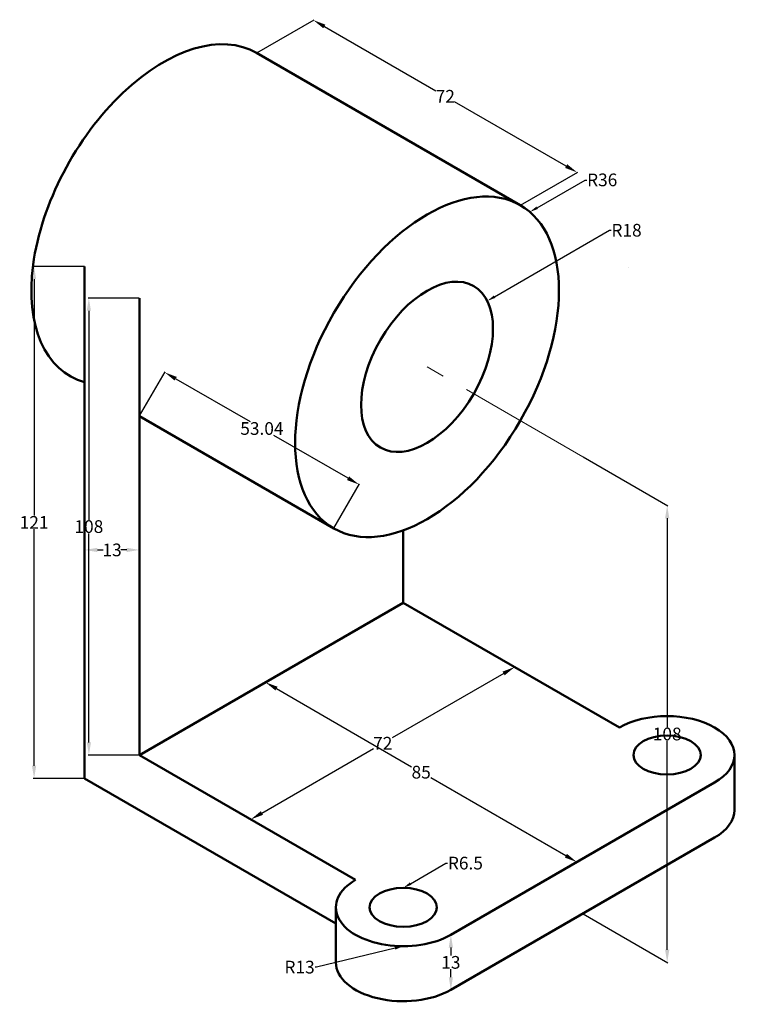
# Model space of a CAD drawing. Units: inches. Extents: x -9 to 160, y -49 to 184.
import ezdxf
from ezdxf import colors
from ezdxf.entities.mleader import LeaderData, LeaderLine
from ezdxf.math import Vec2, Vec3

# ---------------------------------------------------------------- set-up
doc = ezdxf.new("R2010")
doc.units = ezdxf.units.IN
doc.header["$MEASUREMENT"] = 0
doc.linetypes.add('CENTER', pattern=[50.8, 31.75, -6.35, 6.35, -6.35])
for name, color, linetype, lineweight in [('M-CNTR', 1, 'CENTER', 18), ('M-CONS', 8, 'Continuous', 13), ('M-DIMS', 2, 'Continuous', 25), ('M-OUTL', 7, 'Continuous', 50)]:
    doc.layers.add(name, color=color, linetype=linetype, lineweight=lineweight)
doc.styles.get("Standard").update_dxf_attribs({"font": 'arial.ttf'})
doc.dimstyles.get("Standard").update_dxf_attribs({"dimtxt": 3, "dimasz": 3, "dimexe": 0.18, "dimexo": 0.0625, "dimgap": 0.09, "dimtad": 0, "dimtih": 1, "dimtoh": 1, "dimdec": 0, "dimzin": 0, "dimdsep": 46, "dimtxsty": 'Standard', "dimcen": 3, "dimadec": 0, "dimazin": 0, "dimtfac": 1, "dimtdec": 0, "dimtofl": 0, "dimtmove": 0, "dimatfit": 3, "dimfxl": 1, "dimtolj": 1, "dimtzin": 0, "dimarcsym": 0})

# ---------------------------------------------------------------- blocks, each defined once
blk = doc.blocks.new('*D1')
at = {"layer": 'Defpoints', "color": 0, "transparency": 16777216}
for p in [(81.18, 45.91), (107.52, 30.71), (18.82, 9.91)]:
    blk.add_point(p, dxfattribs=at)
at = {"layer": 'M-DIMS', "color": 0, "lineweight": -2, "transparency": 16777216}
for p, q in [((81.24, 45.88), (107.7, 30.6)), ((104.92, 29.21), (78.55, 13.98)), ((18.89, 9.88), (45.35, -5.4)), ((47.76, -3.79), (74.13, 11.43))]:
    blk.add_line(p, q, dxfattribs=at)
at = {"layer": 'M-DIMS', "color": 0, "transparency": 16777216}
for points in [[(104.67, 29.64), (105.17, 28.77), (107.52, 30.71)], [(47.51, -3.36), (48.01, -4.23), (45.17, -5.29)]]:
    blk.add_solid(points, dxfattribs=at)
at = {"layer": 'M-DIMS', "color": 0, "transparency": 16777216, "insert": (76.34, 12.71), "char_height": 3, "attachment_point": 5}
blk.add_mtext('\\A1;72', dxfattribs=at)
blk = doc.blocks.new('*D2')
at = {"layer": 'Defpoints', "color": 0, "transparency": 16777216}
for p in [(92.44, -32.59), (92.44, -45.59), (92.44, -45.59)]:
    blk.add_point(p, dxfattribs=at)
at = {"layer": 'M-DIMS', "color": 0, "lineweight": -2, "transparency": 16777216}
for p, q in [((92.37, -32.59), (92.26, -32.59)), ((92.44, -35.59), (92.44, -37.46)), ((92.44, -42.59), (92.44, -40.71)), ((92.37, -45.59), (92.26, -45.59))]:
    blk.add_line(p, q, dxfattribs=at)
at = {"layer": 'M-DIMS', "color": 0, "transparency": 16777216}
for points in [[(91.94, -35.59), (92.94, -35.59), (92.44, -32.59)], [(91.94, -42.59), (92.94, -42.59), (92.44, -45.59)]]:
    blk.add_solid(points, dxfattribs=at)
at = {"layer": 'M-DIMS', "color": 0, "transparency": 16777216, "insert": (92.44, -39.09), "char_height": 3, "attachment_point": 5}
blk.add_mtext('\\A1;13', dxfattribs=at)
blk = doc.blocks.new('*D3')
at = {"layer": 'Defpoints', "color": 0, "transparency": 16777216}
for p in [(5.87, 58.39), (18.82, 58.39), (18.82, 58.39)]:
    blk.add_point(p, dxfattribs=at)
at = {"layer": 'M-DIMS', "color": 0, "lineweight": -2, "transparency": 16777216}
for p, q in [((5.87, 58.45), (5.87, 58.57)), ((8.87, 58.39), (10.25, 58.39)), ((15.82, 58.39), (14.45, 58.39)), ((18.82, 58.45), (18.82, 58.57))]:
    blk.add_line(p, q, dxfattribs=at)
at = {"layer": 'M-DIMS', "color": 0, "transparency": 16777216}
for points in [[(8.87, 58.89), (8.87, 57.89), (5.87, 58.39)], [(15.82, 58.89), (15.82, 57.89), (18.82, 58.39)]]:
    blk.add_solid(points, dxfattribs=at)
at = {"layer": 'M-DIMS', "color": 0, "transparency": 16777216, "insert": (12.35, 58.39), "char_height": 3, "attachment_point": 5}
blk.add_mtext('\\A1;13', dxfattribs=at)
blk = doc.blocks.new('*D4')
at = {"layer": 'Defpoints', "color": 0, "transparency": 16777216}
for p in [(23.93, 12.86), (122.23, -15.39), (97.55, -29.64)]:
    blk.add_point(p, dxfattribs=at)
at = {"layer": 'M-DIMS', "color": 0, "lineweight": -2, "transparency": 16777216}
for p, q in [((24, 12.9), (48.8, 27.22)), ((51.22, 25.61), (83.17, 7.16)), ((119.63, -13.89), (87.68, 4.56)), ((97.61, -29.6), (122.41, -15.28))]:
    blk.add_line(p, q, dxfattribs=at)
at = {"layer": 'M-DIMS', "color": 0, "transparency": 16777216}
for points in [[(51.47, 26.05), (50.97, 25.18), (48.62, 27.11)], [(119.88, -13.45), (119.38, -14.32), (122.23, -15.39)]]:
    blk.add_solid(points, dxfattribs=at)
at = {"layer": 'M-DIMS', "color": 0, "transparency": 16777216, "insert": (85.42, 5.86), "char_height": 3, "attachment_point": 5}
blk.add_mtext('\\A1;85', dxfattribs=at)
blk = doc.blocks.new('*D5')
at = {"layer": 'Defpoints', "color": 0, "transparency": 16777216}
for p in [(123.61, 80.41), (123.61, -27.59), (143.57, -39.11)]:
    blk.add_point(p, dxfattribs=at)
at = {"layer": 'M-DIMS', "color": 0, "lineweight": -2, "transparency": 16777216}
for p, q in [((123.68, 80.38), (143.75, 68.79)), ((143.57, 65.89), (143.57, 16.51)), ((143.57, -36.11), (143.57, 13.27)), ((123.68, -27.62), (143.75, -39.21))]:
    blk.add_line(p, q, dxfattribs=at)
at = {"layer": 'M-DIMS', "color": 0, "transparency": 16777216}
for points in [[(143.07, 65.89), (144.07, 65.89), (143.57, 68.89)], [(143.07, -36.11), (144.07, -36.11), (143.57, -39.11)]]:
    blk.add_solid(points, dxfattribs=at)
at = {"layer": 'M-DIMS', "color": 0, "transparency": 16777216, "insert": (143.57, 14.89), "char_height": 3, "attachment_point": 5}
blk.add_mtext('\\A1;108', dxfattribs=at)
blk = doc.blocks.new('*D6')
at = {"layer": 'Defpoints', "color": 0, "transparency": 16777216}
for p in [(59.94, 183.61), (46.5, 175.85), (108.85, 139.85)]:
    blk.add_point(p, dxfattribs=at)
at = {"layer": 'M-DIMS', "color": 0, "lineweight": -2, "transparency": 16777216}
for p, q in [((46.56, 175.88), (60.12, 183.71)), ((62.54, 182.11), (88.91, 166.88)), ((119.7, 149.11), (93.33, 164.33)), ((108.92, 139.88), (122.48, 147.71))]:
    blk.add_line(p, q, dxfattribs=at)
at = {"layer": 'M-DIMS', "color": 0, "transparency": 16777216}
for points in [[(62.79, 182.54), (62.29, 181.68), (59.94, 183.61)], [(119.95, 149.54), (119.45, 148.68), (122.3, 147.61)]]:
    blk.add_solid(points, dxfattribs=at)
at = {"layer": 'M-DIMS', "color": 0, "transparency": 16777216, "insert": (91.12, 165.61), "char_height": 3, "attachment_point": 5}
blk.add_mtext('\\A1;72', dxfattribs=at)
blk = doc.blocks.new('*D7')
at = {"layer": 'Defpoints', "color": 0, "transparency": 16777216}
for p in [(-6.08, 125.39), (5.87, 125.39), (5.87, 4.39)]:
    blk.add_point(p, dxfattribs=at)
at = {"layer": 'M-DIMS', "color": 0, "lineweight": -2, "transparency": 16777216}
for p, q in [((5.81, 125.39), (-6.26, 125.39)), ((-6.08, 122.39), (-6.08, 66.49)), ((-6.08, 7.39), (-6.08, 63.3)), ((5.81, 4.39), (-6.26, 4.39))]:
    blk.add_line(p, q, dxfattribs=at)
at = {"layer": 'M-DIMS', "color": 0, "transparency": 16777216}
for points in [[(-6.58, 122.39), (-5.58, 122.39), (-6.08, 125.39)], [(-6.58, 7.39), (-5.58, 7.39), (-6.08, 4.39)]]:
    blk.add_solid(points, dxfattribs=at)
at = {"layer": 'M-DIMS', "color": 0, "transparency": 16777216, "insert": (-6.08, 64.89), "char_height": 3, "attachment_point": 5}
blk.add_mtext('\\A1;121', dxfattribs=at)
blk = doc.blocks.new('*D8')
at = {"layer": 'Defpoints', "color": 0, "transparency": 16777216}
for p in [(6.87, 117.91), (18.82, 117.91), (18.82, 9.91)]:
    blk.add_point(p, dxfattribs=at)
at = {"layer": 'M-DIMS', "color": 0, "lineweight": -2, "transparency": 16777216}
for p, q in [((18.76, 117.91), (6.69, 117.91)), ((6.87, 114.91), (6.87, 65.54)), ((6.87, 12.91), (6.87, 62.29)), ((18.76, 9.91), (6.69, 9.91))]:
    blk.add_line(p, q, dxfattribs=at)
at = {"layer": 'M-DIMS', "color": 0, "transparency": 16777216}
for points in [[(6.37, 114.91), (7.37, 114.91), (6.87, 117.91)], [(6.37, 12.91), (7.37, 12.91), (6.87, 9.91)]]:
    blk.add_solid(points, dxfattribs=at)
at = {"layer": 'M-DIMS', "color": 0, "transparency": 16777216, "insert": (6.87, 63.91), "char_height": 3, "attachment_point": 5}
blk.add_mtext('\\A1;108', dxfattribs=at)
blk = doc.blocks.new('*D9')
at = {"layer": 'Defpoints', "color": 0, "transparency": 16777216}
for p in [(18.82, 90), (70.74, 73.83), (64.76, 63.48)]:
    blk.add_point(p, dxfattribs=at)
at = {"layer": 'M-DIMS', "color": 0, "lineweight": -2, "transparency": 16777216}
for p, q in [((18.86, 90.06), (24.89, 100.51)), ((27.4, 98.85), (44.96, 88.71)), ((68.14, 75.33), (50.58, 85.47)), ((64.79, 63.53), (70.83, 73.98))]:
    blk.add_line(p, q, dxfattribs=at)
at = {"layer": 'M-DIMS', "color": 0, "transparency": 16777216}
for points in [[(27.65, 99.28), (27.15, 98.42), (24.8, 100.35)], [(68.39, 75.76), (67.89, 74.9), (70.74, 73.83)]]:
    blk.add_solid(points, dxfattribs=at)
at = {"layer": 'M-DIMS', "color": 0, "transparency": 16777216, "insert": (47.77, 87.09), "char_height": 3, "attachment_point": 5}
blk.add_mtext('\\A1;53.04', dxfattribs=at)

msp = doc.modelspace()

# ---------------------------------------------------------------- linework, layer by layer
at = {"layer": 'M-CNTR'}
msp.add_line((123.614, 80.414), (86.808, 101.664), dxfattribs=at)
at = {"layer": 'M-CONS'}
msp.add_line((134.401, 125.097), (134.401, 125.097), dxfattribs=at)
at = {"layer": 'M-OUTL'}
for p, q in [((108.853, 139.847), (46.5, 175.847)), ((5.873, 97.48), (5.873, 125.392)), ((18.825, 9.914), (18.825, 117.914)), ((5.873, 4.392), (5.873, 112.392)), ((64.763, 63.48), (18.825, 90.002)), ((81.179, 45.914), (81.179, 63.005)), ((18.825, 9.914), (81.179, 45.914)), ((81.179, 45.914), (132.274, 16.414)), ((18.825, 9.914), (69.92, -19.586)), ((159.454, 9.914), (159.454, -3.086)), ((5.873, 4.392), (65.257, -29.894)), ((92.437, -32.586), (154.791, 3.414)), ((92.437, -45.586), (154.791, -9.586)), ((65.257, -39.086), (65.257, -26.086))]:
    msp.add_line(p, q, dxfattribs=at)
for centre, major_axis, start_param, end_param in [((24.454, 137.664), (-22.045, -38.184), 3.1415927, 6.4300784), ((143.533, 9.914), (-15.922, 0), 2.3561945, 5.4977871), ((143.533, -3.086), (-15.922, 0), 2.3561945, 3.1415927), ((81.179, -26.086), (-15.922, 0), 5.4977871, 8.6393798), ((81.179, -39.086), (-15.922, 0), 6.2831853, 8.6393798)]:
    msp.add_ellipse(centre, major_axis=major_axis, ratio=0.5773503, start_param=start_param, end_param=end_param, dxfattribs=at)
for centre, major_axis in [((86.808, 101.664), (-22.045, -38.184)), ((86.808, 101.664), (-11.023, -19.092)), ((143.533, 9.914), (-7.961, 0)), ((81.179, -26.086), (-7.961, 0))]:
    msp.add_ellipse(centre, major_axis=major_axis, ratio=0.5773503, dxfattribs=at)

# ---------------------------------------------------------------- dimensions: what is measured, and where the dimension line sits
at = {"layer": 'M-DIMS'}
for p1, p2, distance, picture, middle in [((108.853, 139.847), (46.5, 175.847), -13.442, '*D6', (91.119, 165.608)), ((123.614, 80.414), (123.614, -27.586), 19.961, '*D5', (143.575, 14.889)), ((5.873, 58.392), (18.825, 58.392), 0, '*D3', (12.349, 58.392)), ((18.825, 9.914), (81.179, 45.914), -26.34, '*D1', (76.342, 12.706)), ((23.935, 12.864), (97.547, -29.636), 24.682, '*D4', (85.423, 5.864)), ((92.437, -32.586), (92.437, -45.586), 0, '*D2', (92.437, -39.086))]:
    dim = msp.add_aligned_dim(p1=p1, p2=p2, distance=distance, dimstyle='Standard', override={"dimclrd": 0, "dimclre": 0, "dimclrt": 0}, dxfattribs=at)
    dim.commit()
    dim.dimension.update_dxf_attribs({"geometry": picture, "text_midpoint": middle})
for base, p1, p2, angle, override, picture, middle in [((-6.077, 125.392), (5.873, 4.392), (5.873, 125.392), 90, {"dimdec": 0, "dimlfac": 1, "dimrnd": 0, "dimzin": 0, "dimdsep": 46, "dimlunit": 2}, '*D7', (-6.077, 64.892)), ((6.875, 117.914), (18.825, 9.914), (18.825, 117.914), 90, {"dimdec": 0, "dimlfac": 1, "dimrnd": 0, "dimzin": 0, "dimdsep": 46, "dimlunit": 2}, '*D8', (6.875, 63.914)), ((70.738, 73.829), (18.825, 90.002), (64.763, 63.48), 330, {"dimdec": 2, "dimlfac": 1, "dimrnd": 0, "dimzin": 0, "dimdsep": 46, "dimlunit": 2}, '*D9', (47.769, 87.09))]:
    dim = msp.add_linear_dim(base=base, p1=p1, p2=p2, angle=angle, dimstyle='Standard', override=override, dxfattribs=at)
    dim.commit()
    dim.dimension.update_dxf_attribs({"geometry": picture, "text_midpoint": middle})

# ---------------------------------------------------------------- leaders
ml = msp.add_multileader_mtext('Standard', dxfattribs=at)
ml.set_content('R36', color=256)
ml.set_leader_properties()
ml.build(insert=Vec2(0, 0))
ml.multileader.update_dxf_attribs({"dogleg_length": 0.36, "arrow_head_size": 2})
ctx = ml.context
ctx.base_point, ctx.char_height, ctx.arrow_head_size, ctx.landing_gap_size, ctx.plane_origin = Vec3(124.548, 145.822), 3, 2, 0.09, Vec3(111.092, 138.261)
notes = []
notes.append((ctx, [(0, (1, 1, 0), (124.188, 145.822), (1, 0), 0.36, [(0, [(111.092, 138.261)], 0, [])])]))
ctx.mtext.insert, ctx.mtext.flow_direction = Vec3(124.638, 147.349), 5
ml = msp.add_multileader_mtext('Standard', dxfattribs=at)
ml.set_content('R18', color=256)
ml.set_leader_properties()
ml.build(insert=Vec2(0, 0))
ml.multileader.update_dxf_attribs({"dogleg_length": 0.36, "arrow_head_size": 2})
ctx = ml.context
ctx.base_point, ctx.char_height, ctx.arrow_head_size, ctx.landing_gap_size, ctx.plane_origin = Vec3(130.303, 133.929), 3, 2, 0.09, Vec3(101.033, 117.238)
notes.append((ctx, [(0, (1, 1, 0), (129.943, 133.929), (1, 0), 0.36, [(0, [(101.033, 117.238)], 0, [])])]))
ctx.mtext.insert, ctx.mtext.flow_direction = Vec3(130.393, 135.454), 5
ml = msp.add_multileader_mtext('Standard', dxfattribs=at)
ml.set_content('R6.5', color=256)
ml.set_leader_properties()
ml.build(insert=Vec2(0, 0))
ml.multileader.update_dxf_attribs({"dogleg_length": 0.36, "arrow_head_size": 2})
ctx = ml.context
ctx.base_point, ctx.char_height, ctx.arrow_head_size, ctx.landing_gap_size, ctx.plane_origin = Vec3(91.645, -15.655), 3, 2, 0.09, Vec3(81.179, -21.49)
notes.append((ctx, [(0, (1, 1, 0), (91.285, -15.655), (1, 0), 0.36, [(0, [(81.179, -21.49)], 0, [])])]))
ctx.mtext.insert, ctx.mtext.flow_direction = Vec3(91.735, -14.13), 5
ml = msp.add_multileader_mtext('Standard', dxfattribs=at)
ml.set_content('R13', color=256)
ml.set_leader_properties()
ml.build(insert=Vec2(0, 0))
ml.multileader.update_dxf_attribs({"dogleg_length": 0.36, "arrow_head_size": 2})
ctx = ml.context
ctx.base_point, ctx.char_height, ctx.arrow_head_size, ctx.landing_gap_size, ctx.plane_origin = Vec3(52.991, -40.239), 3, 2, 0.09, Vec3(81.179, -35.279)
ctx.text_align_type = 2
notes.append((ctx, [(0, (1, 1, 0), (60.699, -40.239), (-1, 0), 0.36, [(0, [(81.179, -35.279)], 0, [])])]))
ctx.mtext.insert, ctx.mtext.alignment, ctx.mtext.flow_direction = Vec3(60.249, -38.713), 3, 5
for ctx, leaders in notes:
    for number, flags, end, landing, length, lines in leaders:
        leader = LeaderData()
        leader.index, (leader.has_last_leader_line, leader.has_dogleg_vector, leader.attachment_direction) = number, flags
        leader.last_leader_point, leader.dogleg_vector, leader.dogleg_length = Vec3(end), Vec3(landing), length
        for number, points, colour, breaks in lines:
            line = LeaderLine()
            line.index, line.vertices, line.color, line.breaks = number, Vec3.list(points), colors.encode_raw_color(colour), breaks
            leader.lines.append(line)
        ctx.leaders.append(leader)

doc.saveas('drawing.dxf')
